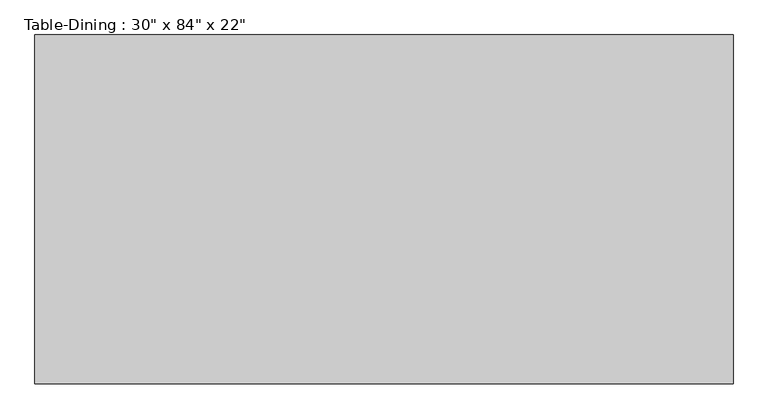
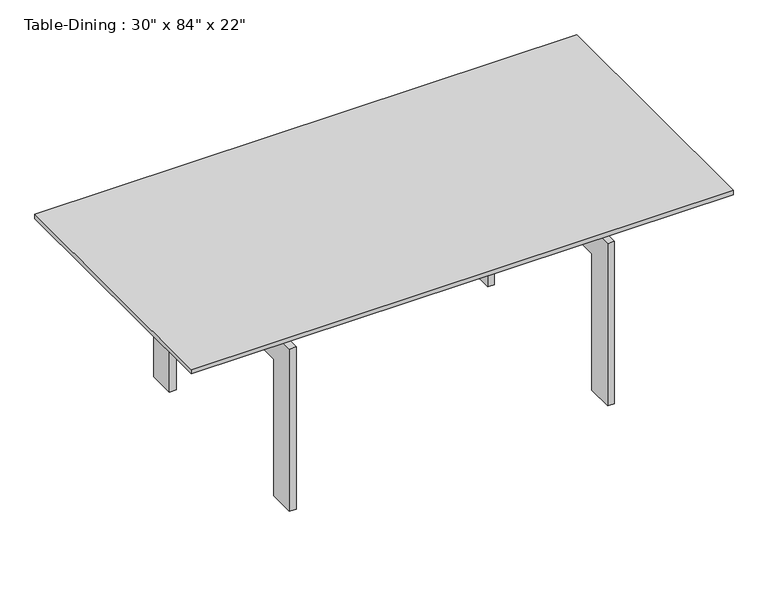
"""IFC4 building model written with IfcOpenShell, lengths in millimetres: furniture geometry."""

from ifc_helpers import new_model, si_unit, frame, origin, place, context, project, spatial, polyline, outline, extrude, source, transform, mapped, element, save


def furniture_37c8c8f5(model_context):
    return source(origin(), model_context, "Body", "SweptSolid", [
        extrude(outline(polyline([(678.6657667, 297.7823857), (678.6657667, 272.3823857), (-642.1342333, 272.3823857), (-642.1342333, 297.7823857), (678.6657667, 297.7823857)])), frame((0.0, 0.0, 482.6), z_axis=(0.0, 0.0, 1.0), x_axis=(1.0, 0.0, 0.0)), (0.0, 0.0, 1.0), 63.5),
        extrude(outline(polyline([(678.6657667, -82.5889222), (678.6657667, -107.9889222), (-642.1342333, -107.9889222), (-642.1342333, -82.5889222), (678.6657667, -82.5889222)])), frame((0.0, 0.0, 482.6), z_axis=(0.0, 0.0, 1.0), x_axis=(1.0, 0.0, 0.0)), (0.0, 0.0, 1.0), 63.5),
        extrude(outline(polyline([(425.4110778, 0.0), (349.2110778, 0.0), (349.2110778, 406.4), (-158.7889222, 406.4), (-158.7889222, 0.0), (-234.9889222, 0.0), (-234.9889222, 482.6), (425.4110778, 482.6), (425.4110778, 0.0)])), frame((456.4157667, 0.0, 0.0), z_axis=(1.0, 0.0, 0.0), x_axis=(0.0, 1.0, 0.0)), (0.0, 0.0, 1.0), 19.05),
        extrude(outline(polyline([(425.4110778, 482.6), (425.4110778, 0.0), (349.2110778, 0.0), (349.2110778, 406.4), (-158.7889222, 406.4), (-158.7889222, 0.0), (-234.9889222, 0.0), (-234.9889222, 482.6), (425.4110778, 482.6)])), frame((-438.9342333, 0.0, 0.0), z_axis=(1.0, 0.0, 0.0), x_axis=(0.0, 1.0, 0.0)), (0.0, 0.0, 1.0), 19.05),
        extrude(outline(polyline([(780.2657667, 476.2110778), (780.2657667, -285.7889222), (-743.7342333, -285.7889222), (-743.7342333, 476.2110778), (780.2657667, 476.2110778)])), frame((0.0, 0.0, 546.1), z_axis=(0.0, 0.0, 1.0), x_axis=(1.0, 0.0, 0.0)), (0.0, 0.0, 1.0), 12.7),
    ])


if __name__ == "__main__":
    model = new_model("IFC4")
    model_context = context("Model", 3, world=origin())
    ifc_project = project(units=[si_unit("LENGTHUNIT", "METRE", prefix="MILLI")], contexts=[model_context])
    site = spatial("IfcSite", under=ifc_project)
    building = spatial("IfcBuilding", under=site)
    placement = place(None, origin())
    furniture_shape = furniture_37c8c8f5(model_context)
    element("IfcFurniture", 1, ObjectType="Table-Dining : 30\" x 84\" x 22\"", at=placement, inside=building, context=model_context, shape_type="MappedRepresentation", body=[
        mapped(furniture_shape, transform((0.0, 0.0, 0.0), x_axis=(1.0, 0.0, 0.0), y_axis=(0.0, 1.0, 0.0), z_axis=(0.0, 0.0, 1.0))),
    ])
    save(model, "model.ifc")

# Revit data of these elements
# Type "Table-Dining : 30\" x 84\" x 22\""
#   Assembly Code = "E2020200"
#   Height = 1' - 10"
#   Length = 5' - 0"
#   Width = 2' - 6"
#   Base Material = Steel, Chrome Plated
#   Top Material = Glass - Clear, Grey
#   Default Elevation = 0
# Element 1 (IfcFurniture, "Table-Dining : 30\" x 84\" x 22\"")
#   Materials on its faces: "Steel, Chrome Plated", "Glass - Clear, Grey"
# Materials
#   "Steel, Chrome Plated": class "Metal", colour RGB 17 17 17, transparency 0, Description = "Chromiuim plated steel", Cost = 0
#   "Glass - Clear, Grey": class "Glass", colour RGB 252 255 255, transparency 0.64
